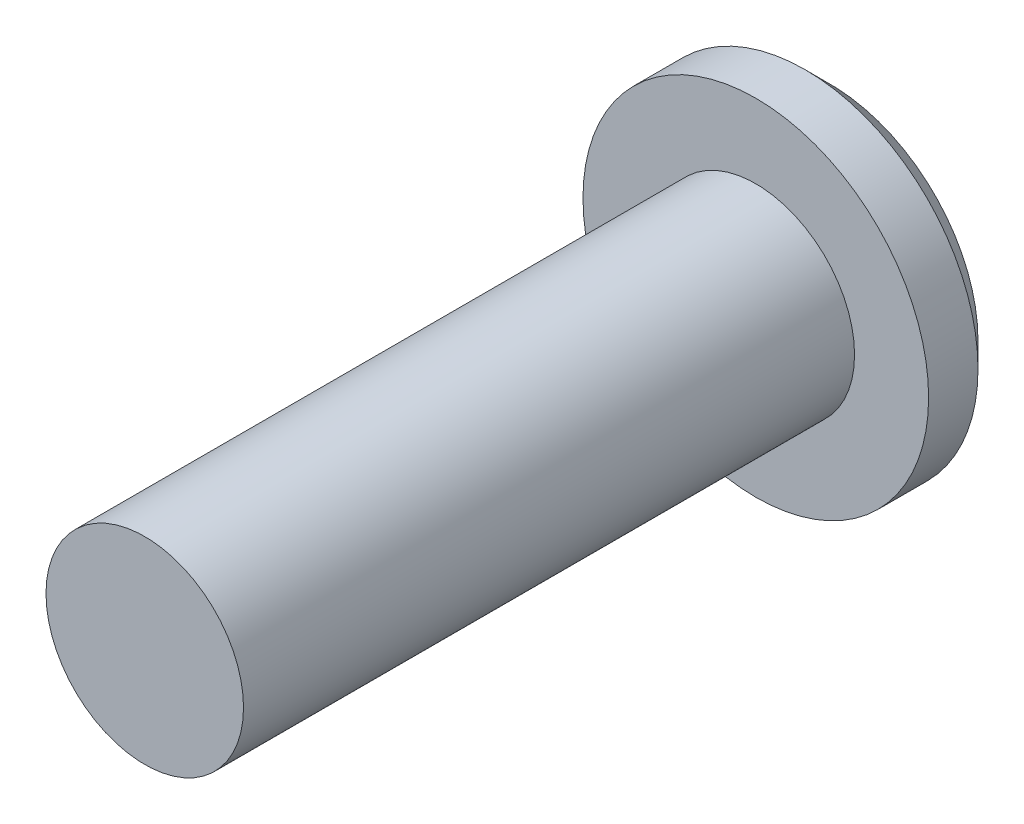
from build123d import *

# Parameters (mm, degrees)
HEAD_PROFILE_14_R      = 7
HEAD_14X3_DEPTH        = 3
SHANK_PROFILE_8_R      = 4
SHANK_8X24_75_DEPTH    = 24.75
HEAD_CHAMFER_1X45_SIZE = 1


with BuildPart() as part:
    # Head Profile Ø14 → Head Ø14x3 (new body)
    with BuildSketch(Plane.XY):
        Circle(HEAD_PROFILE_14_R)
    extrude(amount=HEAD_14X3_DEPTH)

    # Shank Profile Ø8 → Shank Ø8x24.75 (add)
    with BuildSketch(Plane.XY.offset(3)):
        Circle(SHANK_PROFILE_8_R)
    extrude(amount=SHANK_8X24_75_DEPTH)

    # Head Chamfer 1x45°
    head_chamfer_1x45_edges = [part.edges().sort_by_distance(p)[0] for p in [
        (-7, 0, 0),
    ]]
    chamfer(head_chamfer_1x45_edges, length=HEAD_CHAMFER_1X45_SIZE)


solid = part.part
